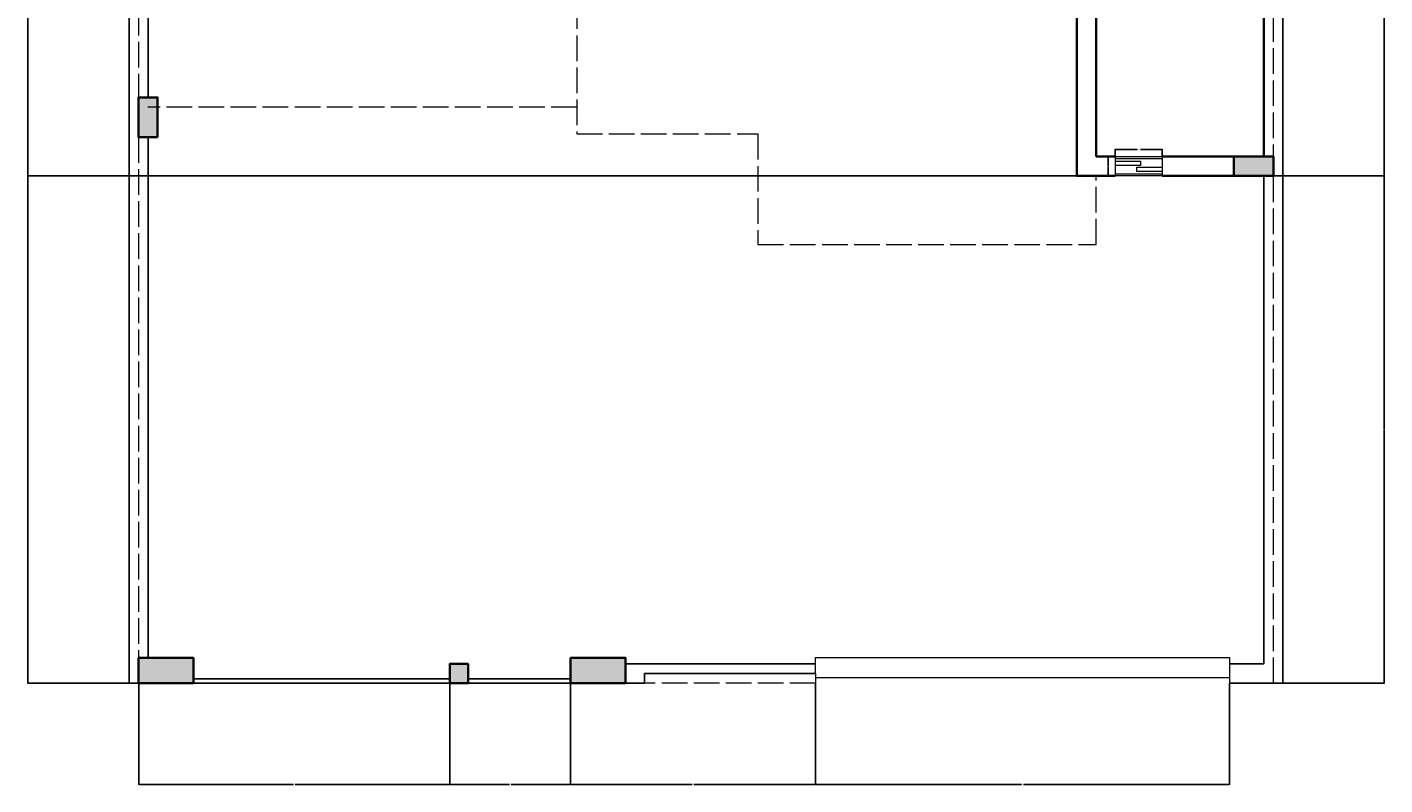
# Model space of a CAD drawing. Units: inches. Extents: x 2711 to 4246, y 540 to 1583.
# Tile 1 of 7: x 2716 to 3351, y 540 to 894. Entities that reach past the tile are written whole.
import ezdxf

# ---------------------------------------------------------------- set-up
doc = ezdxf.new("R2010")
doc.units = ezdxf.units.IN
doc.linetypes.add('ACAD_ISO02W100', pattern=[15, 12, -3])
for name, color, linetype, lineweight in [('A-ANNO-DIMS', 2, 'Continuous', 18), ('A-COLS', 210, 'Continuous', 35), ('A-COLS-PATT', 6, 'Continuous', 13), ('A-FLOR-OVHD', 225, 'ACAD_ISO02W100', 13), ('A-GLAZ', 4, 'Continuous', 18), ('A-WALL', 1, 'Continuous', 35), ('C-PROP-GATE', 32, 'Continuous', 18), ('C-PROP-HIDN', 7, 'ACAD_ISO02W100', 13), ('C-PROP-WALL', 7, 'Continuous', 25)]:
    doc.layers.add(name, color=color, linetype=linetype, lineweight=lineweight)
doc.styles.get("Standard").update_dxf_attribs({"font": 'arial.ttf'})
doc.dimstyles.get("Standard").update_dxf_attribs({"dimtxt": 0.18, "dimasz": 0.18, "dimexe": 0.18, "dimexo": 0.0625, "dimgap": 0.09, "dimtad": 0, "dimtih": 1, "dimtoh": 1, "dimdec": 4, "dimzin": 0, "dimdsep": 46, "dimtxsty": 'Standard', "dimcen": 0.09, "dimadec": 0, "dimazin": 0, "dimtfac": 1, "dimtdec": 4, "dimtofl": 0, "dimtmove": 0, "dimatfit": 3, "dimfxl": 1, "dimtolj": 1, "dimtzin": 0, "dimarcsym": 0})

# ---------------------------------------------------------------- blocks, each defined once
blk = doc.blocks.new('WIN-SLIDER-W04')
for p, q in [((0, 9), (0, 0)), ((0, 9), (22.02, 9)), ((0, 8.1), (22.02, 8.1)), ((0, 6.87), (11.87, 6.87)), ((11.87, 6.87), (11.87, 4.87)), ((22.02, 9), (22.02, 0)), ((11.87, 4.87), (0, 4.87)), ((0, 0.89), (22.02, 0.89)), ((10.15, 2.04), (10.15, 4.04)), ((10.15, 4.04), (22.02, 4.04)), ((22.02, 2.04), (10.15, 2.04)), ((22.02, 0), (0, 0))]:
    blk.add_line(p, q)
blk = doc.blocks.new('*D92')
at = {"layer": 'A-ANNO-DIMS', "color": 0, "lineweight": -2, "transparency": 16777216}
for p, q in [((3225.02, 833.83), (3225.02, 837.25)), ((3225.2, 837.07), (3235.2, 837.07)), ((3246.86, 837.07), (3236.85, 837.07)), ((3247.04, 833.83), (3247.04, 837.25))]:
    blk.add_line(p, q, dxfattribs=at)
at = {"layer": 'A-ANNO-DIMS', "color": 0, "transparency": 16777216}
for points in [[(3225.2, 837.1), (3225.2, 837.04), (3225.02, 837.07)], [(3246.86, 837.1), (3246.86, 837.04), (3247.04, 837.07)]]:
    blk.add_solid(points, dxfattribs=at)
at = {"layer": 'Defpoints', "color": 0, "transparency": 16777216}
for p in [(3225.02, 833.77), (3247.04, 837.07), (3247.04, 833.77)]:
    blk.add_point(p, dxfattribs=at)
at = {"layer": 'A-ANNO-DIMS', "color": 0, "transparency": 16777216, "insert": (3236.03, 837.07), "char_height": 0.18, "attachment_point": 5}
blk.add_mtext('\\A1;W04 22 TYP.', dxfattribs=at)
blk = doc.blocks.new('*D93')
at = {"layer": 'A-ANNO-DIMS', "color": 0, "lineweight": -2, "transparency": 16777216}
for p, q in [((3224.96, 833.77), (3221.54, 833.77)), ((3221.72, 833.59), (3221.72, 829.45)), ((3221.72, 824.95), (3221.72, 829.09)), ((3224.96, 824.77), (3221.54, 824.77))]:
    blk.add_line(p, q, dxfattribs=at)
at = {"layer": 'A-ANNO-DIMS', "color": 0, "transparency": 16777216}
for points in [[(3221.69, 833.59), (3221.75, 833.59), (3221.72, 833.77)], [(3221.69, 824.95), (3221.75, 824.95), (3221.72, 824.77)]]:
    blk.add_solid(points, dxfattribs=at)
at = {"layer": 'Defpoints', "color": 0, "transparency": 16777216}
for p in [(3221.72, 833.77), (3225.02, 833.77), (3225.02, 824.77)]:
    blk.add_point(p, dxfattribs=at)
at = {"layer": 'A-ANNO-DIMS', "color": 0, "transparency": 16777216, "insert": (3221.72, 829.27), "char_height": 0.18, "attachment_point": 5}
blk.add_mtext('\\A1;9 TYP.', dxfattribs=at)
blk = doc.blocks.new('*D95')
at = {"layer": 'A-ANNO-DIMS', "color": 0, "lineweight": -2, "transparency": 16777216}
for p, q in [((2763.43, 1534.95), (2715.94, 1534.95)), ((2716.12, 1534.77), (2716.12, 1061.38)), ((2716.12, 587.63), (2716.12, 1061.02)), ((2763.43, 587.45), (2715.94, 587.45))]:
    blk.add_line(p, q, dxfattribs=at)
at = {"layer": 'A-ANNO-DIMS', "color": 0, "transparency": 16777216}
for points in [[(2716.09, 1534.77), (2716.15, 1534.77), (2716.12, 1534.95)], [(2716.09, 587.63), (2716.15, 587.63), (2716.12, 587.45)]]:
    blk.add_solid(points, dxfattribs=at)
at = {"layer": 'Defpoints', "color": 0, "transparency": 16777216}
for p in [(2716.12, 1534.95), (2763.5, 1534.95), (2763.5, 587.45)]:
    blk.add_point(p, dxfattribs=at)
at = {"layer": 'A-ANNO-DIMS', "color": 0, "transparency": 16777216, "insert": (2716.12, 1061.2), "char_height": 0.18, "attachment_point": 5}
blk.add_mtext('\\A1;947.5', dxfattribs=at)
blk = doc.blocks.new('*D98')
at = {"layer": 'A-ANNO-DIMS', "color": 0, "lineweight": -2, "transparency": 16777216}
for p, q in [((3299.06, 824.75), (3351.05, 824.75)), ((3350.87, 824.57), (3350.87, 706.28)), ((3350.87, 587.63), (3350.87, 705.92)), ((3303.56, 587.45), (3351.05, 587.45))]:
    blk.add_line(p, q, dxfattribs=at)
at = {"layer": 'A-ANNO-DIMS', "color": 0, "transparency": 16777216}
for points in [[(3350.84, 824.57), (3350.9, 824.57), (3350.87, 824.75)], [(3350.84, 587.63), (3350.9, 587.63), (3350.87, 587.45)]]:
    blk.add_solid(points, dxfattribs=at)
at = {"layer": 'Defpoints', "color": 0, "transparency": 16777216}
for p in [(3299, 824.75), (3350.87, 824.75), (3303.5, 587.45)]:
    blk.add_point(p, dxfattribs=at)
at = {"layer": 'A-ANNO-DIMS', "color": 0, "transparency": 16777216, "insert": (3350.87, 706.1), "char_height": 0.18, "attachment_point": 5}
blk.add_mtext('\\A1;237.3', dxfattribs=at)
blk = doc.blocks.new('*D99')
at = {"layer": 'A-ANNO-DIMS', "color": 0, "lineweight": -2, "transparency": 16777216}
for p, q in [((3299.06, 1046.94), (3351.05, 1046.94)), ((3350.87, 1046.76), (3350.87, 936.03)), ((3350.87, 824.93), (3350.87, 935.67)), ((3299.06, 824.75), (3351.05, 824.75))]:
    blk.add_line(p, q, dxfattribs=at)
at = {"layer": 'A-ANNO-DIMS', "color": 0, "transparency": 16777216}
for points in [[(3350.84, 1046.76), (3350.9, 1046.76), (3350.87, 1046.94)], [(3350.84, 824.93), (3350.9, 824.93), (3350.87, 824.75)]]:
    blk.add_solid(points, dxfattribs=at)
at = {"layer": 'Defpoints', "color": 0, "transparency": 16777216}
for p in [(3299, 1046.94), (3350.87, 1046.94), (3299, 824.75)]:
    blk.add_point(p, dxfattribs=at)
at = {"layer": 'A-ANNO-DIMS', "color": 0, "transparency": 16777216, "insert": (3350.87, 935.85), "char_height": 0.18, "attachment_point": 5}
blk.add_mtext('\\A1;222.2', dxfattribs=at)
blk = doc.blocks.new('*D104')
at = {"layer": 'A-ANNO-DIMS', "color": 0, "lineweight": -2, "transparency": 16777216}
for p, q in [((3215.96, 905.77), (2715.94, 905.77)), ((2716.12, 905.59), (2716.12, 865.45)), ((2716.12, 824.95), (2716.12, 865.09)), ((3215.96, 824.77), (2715.94, 824.77))]:
    blk.add_line(p, q, dxfattribs=at)
at = {"layer": 'A-ANNO-DIMS', "color": 0, "transparency": 16777216}
for points in [[(2716.09, 905.59), (2716.15, 905.59), (2716.12, 905.77)], [(2716.09, 824.95), (2716.15, 824.95), (2716.12, 824.77)]]:
    blk.add_solid(points, dxfattribs=at)
at = {"layer": 'Defpoints', "color": 0, "transparency": 16777216}
for p in [(3216.02, 905.77), (2716.12, 824.77), (3216.02, 824.77)]:
    blk.add_point(p, dxfattribs=at)
at = {"layer": 'A-ANNO-DIMS', "color": 0, "transparency": 16777216, "insert": (2716.12, 865.27), "char_height": 0.18, "attachment_point": 5}
blk.add_mtext('\\A1;81', dxfattribs=at)
blk = doc.blocks.new('*D120')
at = {"layer": 'A-ANNO-DIMS', "color": 0, "lineweight": -2, "transparency": 16777216}
for p, q in [((2768, 587.39), (2768, 539.89)), ((2913.6, 587.39), (2913.6, 539.89)), ((2768.18, 540.07), (2840.41, 540.07)), ((2913.42, 540.07), (2841.19, 540.07))]:
    blk.add_line(p, q, dxfattribs=at)
at = {"layer": 'A-ANNO-DIMS', "color": 0, "transparency": 16777216}
for points in [[(2768.18, 540.1), (2768.18, 540.04), (2768, 540.07)], [(2913.42, 540.1), (2913.42, 540.04), (2913.6, 540.07)]]:
    blk.add_solid(points, dxfattribs=at)
at = {"layer": 'Defpoints', "color": 0, "transparency": 16777216}
for p in [(2768, 587.45), (2913.6, 587.45), (2913.6, 540.07)]:
    blk.add_point(p, dxfattribs=at)
at = {"layer": 'A-ANNO-DIMS', "color": 0, "transparency": 16777216, "insert": (2840.8, 540.07), "char_height": 0.18, "attachment_point": 5}
blk.add_mtext('\\A1;145.6', dxfattribs=at)
blk = doc.blocks.new('*D121')
at = {"layer": 'A-ANNO-DIMS', "color": 0, "lineweight": -2, "transparency": 16777216}
for p, q in [((2913.6, 587.39), (2913.6, 539.89)), ((2970.16, 587.39), (2970.16, 539.89)), ((2913.78, 540.07), (2941.49, 540.07)), ((2969.98, 540.07), (2942.28, 540.07))]:
    blk.add_line(p, q, dxfattribs=at)
at = {"layer": 'A-ANNO-DIMS', "color": 0, "transparency": 16777216}
for points in [[(2913.78, 540.1), (2913.78, 540.04), (2913.6, 540.07)], [(2969.98, 540.1), (2969.98, 540.04), (2970.16, 540.07)]]:
    blk.add_solid(points, dxfattribs=at)
at = {"layer": 'Defpoints', "color": 0, "transparency": 16777216}
for p in [(2913.6, 587.45), (2970.16, 587.45), (2970.16, 540.07)]:
    blk.add_point(p, dxfattribs=at)
at = {"layer": 'A-ANNO-DIMS', "color": 0, "transparency": 16777216, "insert": (2941.88, 540.07), "char_height": 0.18, "attachment_point": 5}
blk.add_mtext('\\A1;56.55', dxfattribs=at)
blk = doc.blocks.new('*D122')
at = {"layer": 'A-ANNO-DIMS', "color": 0, "lineweight": -2, "transparency": 16777216}
for p, q in [((2970.16, 587.39), (2970.16, 539.89)), ((3084.77, 587.39), (3084.77, 539.89)), ((2970.34, 540.07), (3027.08, 540.07)), ((3084.59, 540.07), (3027.85, 540.07))]:
    blk.add_line(p, q, dxfattribs=at)
at = {"layer": 'A-ANNO-DIMS', "color": 0, "transparency": 16777216}
for points in [[(2970.34, 540.1), (2970.34, 540.04), (2970.16, 540.07)], [(3084.59, 540.1), (3084.59, 540.04), (3084.77, 540.07)]]:
    blk.add_solid(points, dxfattribs=at)
at = {"layer": 'Defpoints', "color": 0, "transparency": 16777216}
for p in [(2970.16, 587.45), (3084.77, 587.45), (3084.77, 540.07)]:
    blk.add_point(p, dxfattribs=at)
at = {"layer": 'A-ANNO-DIMS', "color": 0, "transparency": 16777216, "insert": (3027.46, 540.07), "char_height": 0.18, "attachment_point": 5}
blk.add_mtext('\\A1;114.6', dxfattribs=at)
blk = doc.blocks.new('*D123')
at = {"layer": 'A-ANNO-DIMS', "color": 0, "lineweight": -2, "transparency": 16777216}
for p, q in [((3084.77, 587.39), (3084.77, 539.89)), ((3278.41, 587.39), (3278.41, 539.89)), ((3084.95, 540.07), (3181.14, 540.07)), ((3278.23, 540.07), (3182.05, 540.07))]:
    blk.add_line(p, q, dxfattribs=at)
at = {"layer": 'A-ANNO-DIMS', "color": 0, "transparency": 16777216}
for points in [[(3084.95, 540.1), (3084.95, 540.04), (3084.77, 540.07)], [(3278.23, 540.1), (3278.23, 540.04), (3278.41, 540.07)]]:
    blk.add_solid(points, dxfattribs=at)
at = {"layer": 'Defpoints', "color": 0, "transparency": 16777216}
for p in [(3084.77, 587.45), (3278.41, 587.45), (3278.41, 540.07)]:
    blk.add_point(p, dxfattribs=at)
at = {"layer": 'A-ANNO-DIMS', "color": 0, "transparency": 16777216, "insert": (3181.59, 540.07), "char_height": 0.18, "attachment_point": 5}
blk.add_mtext('\\A1;193.65', dxfattribs=at)

msp = doc.modelspace()

# ---------------------------------------------------------------- hatches: boundary and pattern name
at = {"layer": 'A-COLS-PATT'}
h = msp.add_hatch(color=256, dxfattribs=at)
h.dxf.hatch_style = 1
h.paths.add_polyline_path([(2767.9955, 1384.9055), (2776.9955, 1384.9055), (2776.9955, 1403.4493), (2767.9955, 1403.4493)])
h.paths.add_polyline_path([(3065.5392, 1394.4493), (3065.5392, 1403.4493), (3046.9955, 1403.4493), (3046.9955, 1394.4493)])
h.paths.add_polyline_path([(3298.9955, 1394.4493), (3298.9955, 1403.4493), (3280.4517, 1403.4493), (3280.4517, 1394.4493)])
h.paths.add_polyline_path([(2767.8485, 1230.0438), (2776.8485, 1230.0353), (2776.8485, 1248.5791), (2767.8485, 1248.5791)])
h.paths.add_polyline_path([(2871.9955, 1229.9493), (2871.9955, 1238.9493), (2863.4422, 1238.9493), (2863.4422, 1229.9531), (2867.4955, 1229.9493)])
h.paths.add_polyline_path([(3055.9955, 1229.9493), (3055.9955, 1238.9493), (3037.4517, 1238.9493), (3037.4517, 1229.9493)])
h.paths.add_polyline_path([(3298.9955, 1229.9493), (3298.9955, 1238.9493), (3280.4517, 1238.9493), (3280.4517, 1229.9493)])
h.paths.add_polyline_path([(2776.8485, 1056.0394), (2767.8485, 1056.0394), (2767.8485, 1037.4957), (2776.8485, 1037.4957)])
h.paths.add_polyline_path([(2973.0214, 1041.7894), (2973.0214, 1037.4957), (2982.0148, 1037.4957), (2982.0148, 1056.0394), (2973.0148, 1056.0394), (2973.0148, 1052.2894), (2973.0214, 1052.2894), (2973.0214, 1047.0394)])
h.paths.add_polyline_path([(3063.0214, 1037.4957), (3063.0214, 1056.0394), (3054.0214, 1056.0394), (3054.0214, 1037.4957)])
h.paths.add_polyline_path([(3294.4955, 1046.9493), (3298.9955, 1046.9493), (3298.9955, 1055.9413), (3280.4517, 1055.9413), (3280.4517, 1046.9493)])
h.paths.add_polyline_path([(2982.0214, 924.0394), (2973.0214, 924.0394), (2973.0214, 905.4957), (2982.0214, 905.4957)])
h.paths.add_polyline_path([(3054.0214, 905.4957), (3063.0214, 905.4957), (3063.0214, 924.0394), (3054.0214, 924.0394)])
h.paths.add_polyline_path([(3216.0214, 905.7675), (3216.0214, 914.7675), (3197.4776, 914.7675), (3197.4776, 905.7675)])
h.paths.add_polyline_path([(2776.8485, 842.8947), (2776.8485, 861.4385), (2767.8485, 861.4385), (2767.8485, 842.8947)])
h.paths.add_polyline_path([(3294.4955, 824.7675), (3298.9955, 824.7498), (3298.9955, 833.7498), (3280.4517, 833.7498), (3280.4517, 824.7675)])
h.paths.add_polyline_path([(2793.6045, 587.4493), (2793.6045, 599.3563), (2767.9955, 599.3563), (2767.9955, 587.4493)])
h.paths.add_polyline_path([(2922.1577, 587.4493), (2922.1577, 596.4493), (2913.6045, 596.4493), (2913.6045, 587.4493)])
h.paths.add_polyline_path([(2995.7668, 587.4493), (2995.7668, 599.3563), (2970.1577, 599.3563), (2970.1577, 587.4493)])

# ---------------------------------------------------------------- linework, layer by layer
at = {"layer": 'A-COLS'}
msp.add_line((2922.1577, 596.4493), (2913.6045, 596.4493), dxfattribs=at)
for points in [[(2776.8485, 842.8947), (2776.8485, 861.4385), (2767.8485, 861.4385), (2767.8485, 842.8947)], [(3298.9955, 833.7498), (3280.4517, 833.7498), (3280.4517, 824.7498), (3298.9955, 824.7498)], [(2767.9955, 599.3563), (2793.6045, 599.3563), (2793.6045, 587.4493), (2767.9955, 587.4493)], [(2970.1577, 599.3563), (2995.7668, 599.3563), (2995.7668, 587.4493), (2970.1577, 587.4493)], [(2913.6045, 587.4493), (2922.1577, 587.4493), (2922.1577, 596.4493), (2913.6045, 596.4493)]]:
    msp.add_lwpolyline(points, close=True, dxfattribs=at)
at = {"layer": 'A-FLOR-OVHD'}
for p, q in [((2973.0214, 905.4957), (2973.0214, 844.38)), ((2973.0214, 856.8749), (2772.3485, 856.8749)), ((2973.0214, 844.38), (3057.7955, 844.38)), ((3057.7955, 844.38), (3057.7955, 792.5892)), ((3216.0214, 792.5892), (3216.0214, 824.7675)), ((3057.7955, 792.5892), (3216.0214, 792.5892))]:
    msp.add_line(p, q, dxfattribs=at)
at = {"layer": 'A-WALL'}
for p, q in [((3294.4955, 1046.9493), (3294.4955, 833.7498)), ((3207.0214, 824.7675), (3207.0214, 905.7675)), ((3216.0214, 905.7675), (3216.0214, 833.7675)), ((3216.0214, 833.7675), (3225.0214, 833.7675)), ((3247.0365, 833.7675), (3294.4955, 833.7675)), ((3216.0214, 824.7675), (3207.0214, 824.7675)), ((3225.0214, 824.7675), (3216.0214, 824.7675)), ((3247.0365, 824.7675), (3294.4955, 824.7675))]:
    msp.add_line(p, q, dxfattribs=at)
at = {"layer": 'C-PROP-GATE'}
for p, q in [((3084.7668, 596.4493), (3084.7668, 599.4493)), ((3084.7668, 599.4493), (3278.4149, 599.4493)), ((3278.4149, 599.4493), (3278.4149, 596.4493)), ((3084.7668, 591.9493), (3084.7668, 596.4493)), ((3084.7668, 591.9493), (3084.7668, 596.4493)), ((3084.7668, 591.9493), (3084.7668, 589.9493)), ((3278.4149, 596.4493), (3278.4149, 591.9493)), ((3278.4149, 591.9493), (3278.4149, 589.9493)), ((3278.4149, 589.9493), (3084.7668, 589.9493)), ((3084.7668, 589.9493), (3084.7668, 587.4493)), ((3278.4149, 589.9493), (3278.4149, 587.4493))]:
    msp.add_line(p, q, dxfattribs=at)
at = {"layer": 'C-PROP-HIDN'}
for p, q in [((3298.9955, 587.4493), (3298.9955, 1530.4493)), ((2767.9955, 1037.4957), (2767.9955, 861.4385)), ((2767.9955, 842.8947), (2767.9955, 587.4493)), ((3084.7668, 591.9493), (3084.7668, 596.4493)), ((3084.7668, 587.4493), (3004.7668, 587.4493))]:
    msp.add_line(p, q, dxfattribs=at)
at = {"layer": 'C-PROP-WALL'}
for p, q in [((2763.4955, 587.4493), (2763.4955, 1530.4493)), ((3303.4955, 1530.4493), (3303.4955, 587.4493)), ((2772.4955, 861.4385), (2772.4955, 1037.4957)), ((2772.4955, 599.3563), (2772.4955, 842.8947)), ((3294.4955, 824.7675), (3294.4955, 596.4493)), ((3084.7668, 596.4493), (2995.7668, 596.4493)), ((3004.7668, 587.4493), (3004.7668, 591.9493)), ((3004.7668, 591.9493), (3084.7668, 591.9493)), ((3294.4955, 596.4493), (3278.4149, 596.4493)), ((2767.9955, 587.4493), (2763.4955, 587.4493)), ((2793.6045, 589.4493), (2913.6045, 589.4493)), ((2793.6045, 587.4493), (2913.6045, 587.4493)), ((2913.6045, 589.4493), (2913.6045, 587.4493)), ((2922.1577, 589.4493), (2970.1577, 589.4493)), ((2922.1577, 587.4493), (2970.1577, 587.4493)), ((2970.1577, 589.4493), (2970.1577, 587.4493)), ((2995.7668, 587.4493), (2998.7668, 587.4493)), ((2998.7668, 587.4493), (3000.7668, 587.4493)), ((3000.7668, 587.4493), (3002.7668, 587.4493)), ((3002.7668, 587.4493), (3004.7668, 587.4493)), ((3298.9955, 587.4493), (3278.4149, 587.4493)), ((3303.4955, 587.4493), (3298.9955, 587.4493))]:
    msp.add_line(p, q, dxfattribs=at)

# ---------------------------------------------------------------- block references
at = {"layer": 'A-GLAZ'}
msp.add_blockref('WIN-SLIDER-W04', (3225.021, 824.768), dxfattribs=at)

# ---------------------------------------------------------------- dimensions: what is measured, and where the dimension line sits
at = {"layer": 'A-ANNO-DIMS'}
for base, p1, p2, override, picture, middle in [((2716.1185, 1534.9493), (2763.4955, 587.4493), (2763.4955, 1534.9493), {"dimdec": 1, "dimlfac": 1, "dimrnd": 0, "dimzin": 0, "dimdsep": 46, "dimlunit": 2}, '*D95', (2716.1185, 1061.1993)), ((3350.8725, 1046.9413), (3298.9955, 824.7498), (3298.9955, 1046.9413), {"dimdec": 1, "dimlfac": 1, "dimrnd": 0, "dimzin": 0, "dimdsep": 46, "dimlunit": 2}, '*D99', (3350.8725, 935.8456)), ((2716.1185, 824.7675), (3216.0214, 905.7675), (3216.0214, 824.7675), {"dimdec": 0, "dimlfac": 1, "dimrnd": 0, "dimzin": 0, "dimdsep": 46, "dimlunit": 2}, '*D104', (2716.1185, 865.2675)), ((3350.8725, 824.7498), (3303.4955, 587.4493), (3298.9955, 824.7498), {"dimdec": 1, "dimlfac": 1, "dimrnd": 0, "dimzin": 0, "dimdsep": 46, "dimlunit": 2}, '*D98', (3350.8725, 706.0995))]:
    dim = msp.add_linear_dim(base=base, p1=p1, p2=p2, angle=90, dimstyle='Standard', override=override, dxfattribs=at)
    dim.commit()
    dim.dimension.update_dxf_attribs({"geometry": picture, "text_midpoint": middle})
dim = msp.add_linear_dim(base=(3221.7191, 833.7675), p1=(3225.0214, 824.7675), p2=(3225.0214, 833.7675), angle=90, text='<> TYP.', dimstyle='Standard', override={"dimdec": 0, "dimlfac": 1, "dimrnd": 0, "dimzin": 0, "dimdsep": 46, "dimlunit": 2}, dxfattribs=at)
dim.commit()
dim.dimension.update_dxf_attribs({"geometry": '*D93', "text_midpoint": (3221.7191, 829.2675)})
dim = msp.add_linear_dim(base=(3247.0365, 837.0698), p1=(3225.0214, 833.7675), p2=(3247.0365, 833.7675), text='W04 <> TYP.', dimstyle='Standard', override={"dimdec": 0, "dimlfac": 1, "dimrnd": 0, "dimzin": 0, "dimdsep": 46, "dimlunit": 2}, dxfattribs=at)
dim.commit()
dim.dimension.update_dxf_attribs({"geometry": '*D92', "text_midpoint": (3236.029, 837.0698)})
for base, p1, p2, override, picture, middle in [((2913.6045, 540.0723), (2767.9955, 587.4493), (2913.6045, 587.4493), {"dimdec": 1, "dimlfac": 1, "dimrnd": 0, "dimzin": 0, "dimdsep": 46, "dimlunit": 2}, '*D120', (2840.8, 540.0723)), ((2970.1577, 540.0723), (2913.6045, 587.4493), (2970.1577, 587.4493), {"dimdec": 2, "dimlfac": 1, "dimrnd": 0, "dimzin": 0, "dimdsep": 46, "dimlunit": 2}, '*D121', (2941.8811, 540.0723)), ((3084.7668, 540.0723), (2970.1577, 587.4493), (3084.7668, 587.4493), {"dimdec": 1, "dimlfac": 1, "dimrnd": 0, "dimzin": 0, "dimdsep": 46, "dimlunit": 2}, '*D122', (3027.4623, 540.0723)), ((3278.4149, 540.0723), (3084.7668, 587.4493), (3278.4149, 587.4493), {"dimdec": 2, "dimlfac": 1, "dimrnd": 0, "dimzin": 0, "dimdsep": 46, "dimlunit": 2}, '*D123', (3181.5909, 540.0723))]:
    dim = msp.add_linear_dim(base=base, p1=p1, p2=p2, dimstyle='Standard', override=override, dxfattribs=at)
    dim.commit()
    dim.dimension.update_dxf_attribs({"geometry": picture, "text_midpoint": middle})

doc.saveas('drawing.dxf')
